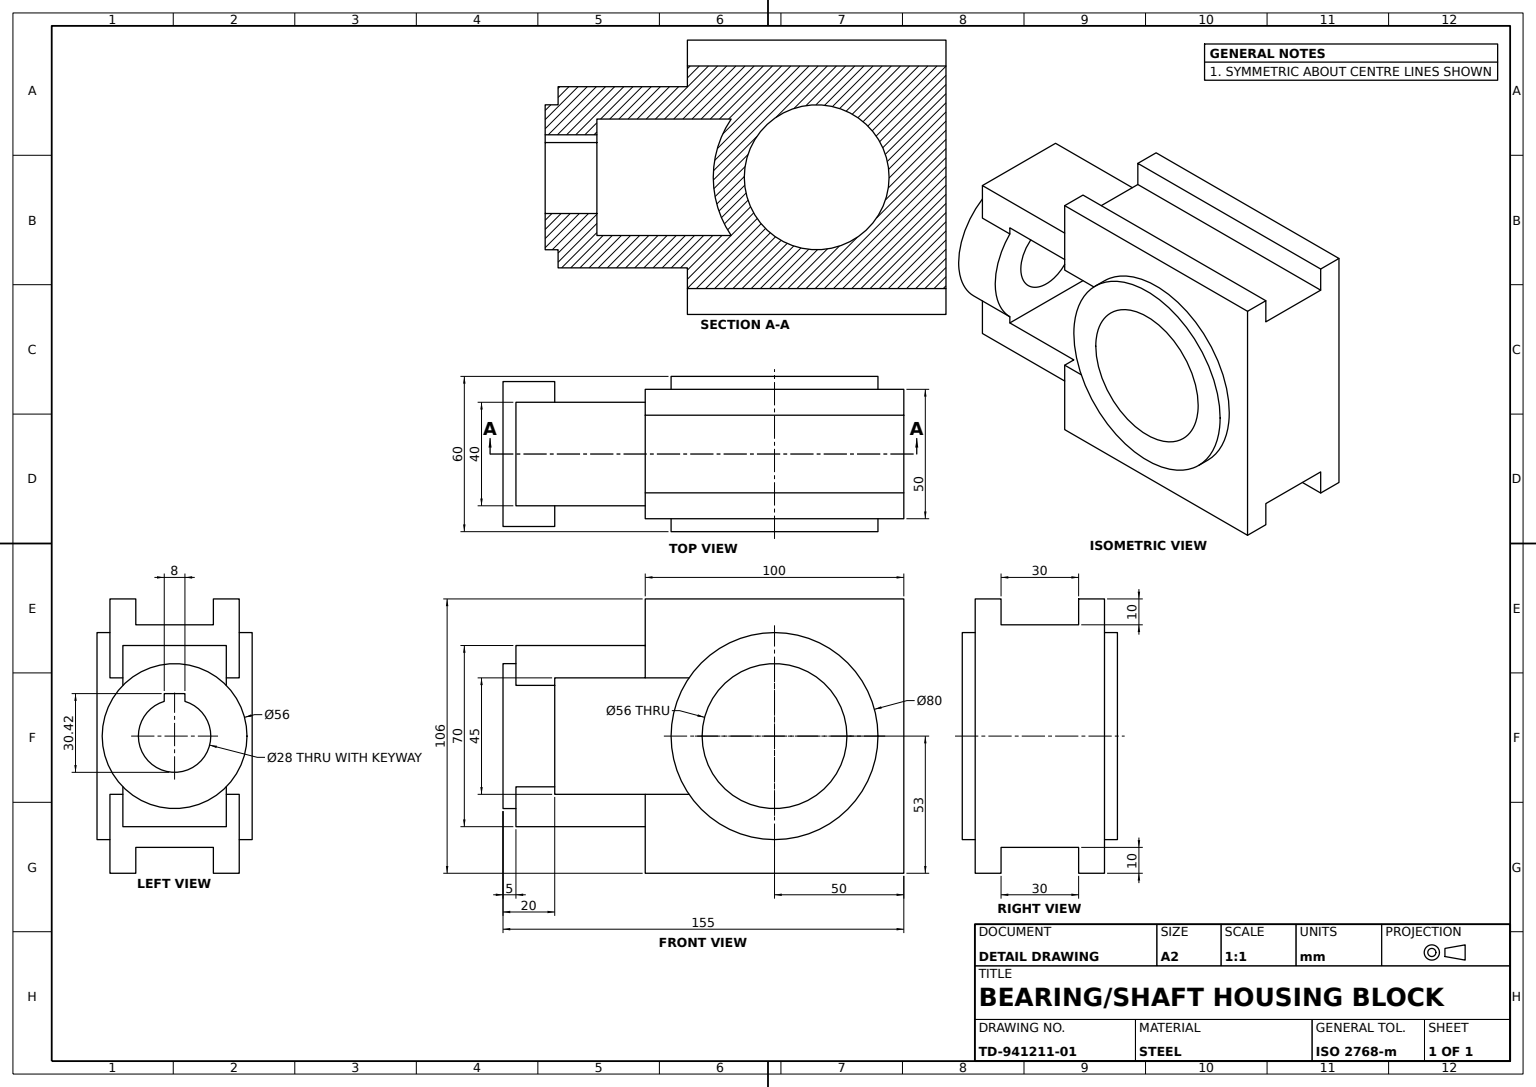
from build123d import *

# Parameters (mm, degrees)
BASE_BLOCK_PROFILE_W         = 100
BASE_BLOCK_PROFILE_H         = 106
BASE_BLOCK_DEPTH             = 25
HOUSING_BOSS_PROFILE_W       = 50
HOUSING_BOSS_PROFILE_H       = 70
HOUSING_BOSS_DEPTH           = 20
GUIDE_KEY_SLOTS_PROFILE_W    = 30
GUIDE_KEY_SLOTS_PROFILE_H    = 10
GUIDE_KEY_SLOTS_DEPTH        = 100
BEARING_BOSS_PROFILE_80_R    = 40
BEARING_BOSS_80_DEPTH        = 30
BEARING_COLLAR_56_DEPTH      = 5
BEARING_COLLAR_56_DEPTH_BACK = 15
BEARING_COLLAR_PROFILE_56_R  = 28
BEARING_BORE_DEPTH           = 122.383689184
BEARING_BORE_DEPTH_BACK      = 122.383689184
BEARING_BORE_PROFILE_R       = 28
BORE_KEYWAY_DEPTH            = 20


with BuildPart() as part:
    # Base Block Profile → Base Block (new, symmetric)
    with BuildSketch(Plane.XY):
        Rectangle(BASE_BLOCK_PROFILE_W, BASE_BLOCK_PROFILE_H)
    extrude(amount=BASE_BLOCK_DEPTH, both=True)

    # Housing Boss Profile → Housing Boss (add, symmetric)
    with BuildSketch(Plane.XY):
        with Locations((-75, 0)):
            Rectangle(HOUSING_BOSS_PROFILE_W, HOUSING_BOSS_PROFILE_H)
    extrude(amount=HOUSING_BOSS_DEPTH, both=True)

    # Guide Key Slots Profile → Guide Key Slots (cut)
    with BuildSketch(Plane.ZY.offset(50)):
        with Locations((0, 48)):
            Rectangle(GUIDE_KEY_SLOTS_PROFILE_W, GUIDE_KEY_SLOTS_PROFILE_H)
        with Locations((0, -48)):
            Rectangle(GUIDE_KEY_SLOTS_PROFILE_W, GUIDE_KEY_SLOTS_PROFILE_H)
    extrude(amount=-GUIDE_KEY_SLOTS_DEPTH, mode=Mode.SUBTRACT)

    # Bearing Boss Profile Ø80 → Bearing Boss Ø80 (add, symmetric)
    with BuildSketch(Plane.XY):
        with Locations(Location((0, 0, 0), (0, 0, 180))):
            Circle(BEARING_BOSS_PROFILE_80_R)
    extrude(amount=BEARING_BOSS_80_DEPTH, both=True)

    # Bearing Collar Profile Ø56 → Bearing Collar Ø56 (add, two sides: drawn at the far end of the back side and taken through both)
    with BuildSketch(Plane.ZY.offset(100).offset(-BEARING_COLLAR_56_DEPTH_BACK)):
        with Locations(Location((0, 0, 0), (0, 0, 224.415308597))):
            Circle(BEARING_COLLAR_PROFILE_56_R)
    extrude(amount=BEARING_COLLAR_56_DEPTH + BEARING_COLLAR_56_DEPTH_BACK)

    # Bearing Bore Profile → Bearing Bore (cut, two sides: drawn at the far end of the back side and taken through both)
    with BuildSketch(Plane.XY.offset(-BEARING_BORE_DEPTH_BACK)):
        Circle(BEARING_BORE_PROFILE_R)
        with BuildLine():
            Line((-85, 22.5), (-33.071891388, 22.5))
            ThreePointArc((-33.071891388, 22.5), (-40, 0), (-33.071891388, -22.5))
            Line((-33.071891388, -22.5), (-85, -22.5))
            Line((-85, -22.5), (-85, 22.5))
        make_face()
    extrude(amount=BEARING_BORE_DEPTH + BEARING_BORE_DEPTH_BACK, mode=Mode.SUBTRACT)

    # Bore Keyway Profile → Bore Keyway (cut)
    with BuildSketch(Plane.ZY.offset(105)):
        with BuildLine():
            Line((-4, 13.416407865), (-4, 16.416407865))
            Line((-4, 16.416407865), (4, 16.416407865))
            Line((4, 16.416407865), (4, 13.416407865))
            ThreePointArc((4, 13.416407865), (0, -14), (-4, 13.416407865))
        make_face()
    extrude(amount=-BORE_KEYWAY_DEPTH, mode=Mode.SUBTRACT)


solid = part.part
